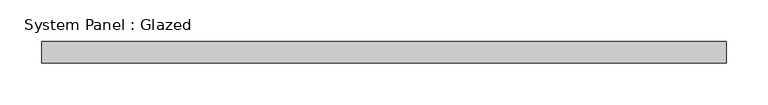
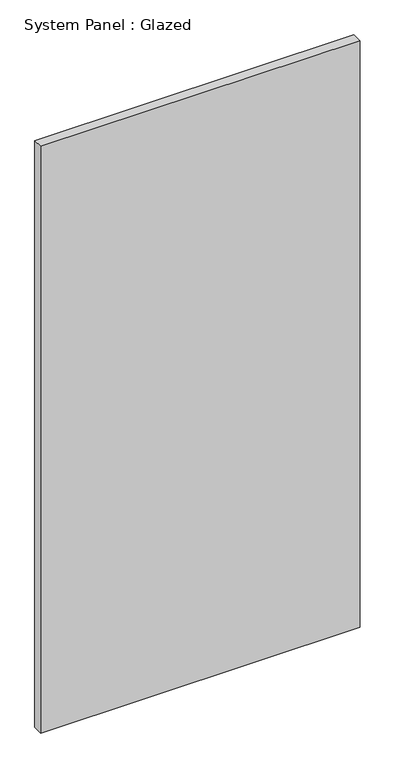
"""IFC4 building model written with IfcOpenShell, lengths in millimetres: plate geometry, System Panel : Glazed."""

from ifc_helpers import new_model, si_unit, origin, origin_with_axes, place, context, project, spatial, polyline, outline, extrude, source, transform, mapped, element, save


def system_panel_glazed_30877d7e(model_context):
    return source(origin(), model_context, "Body", "SweptSolid", [
        extrude(outline(polyline([(409.575, 19.05), (-409.575, 19.05), (-409.575, 44.45), (409.575, 44.45), (409.575, 19.05)])), origin_with_axes(), (0.0, 0.0, 1.0), 1590.1019301),
    ])


if __name__ == "__main__":
    model = new_model("IFC4")
    model_context = context("Model", 3, world=origin())
    ifc_project = project(units=[si_unit("LENGTHUNIT", "METRE", prefix="MILLI")], contexts=[model_context])
    site = spatial("IfcSite", under=ifc_project)
    building = spatial("IfcBuilding", under=site)
    placement = place(None, origin())
    system_panel_glazed_shape = system_panel_glazed_30877d7e(model_context)
    element("IfcPlate", 1, ObjectType="System Panel : Glazed", at=placement, inside=building, context=model_context, shape_type="MappedRepresentation", body=[
        mapped(system_panel_glazed_shape, transform((0.0, 0.0, 0.0), x_axis=(1.0, 0.0, 0.0), y_axis=(0.0, 1.0, 0.0), z_axis=(0.0, 0.0, 1.0))),
    ])
    save(model, "model.ifc")

# Revit data of these elements
# Type "System Panel : Glazed"
#   Construction Type Id = "GSP4R"
#   Analytic Construction = "1/8 in Pilkington single glazing"
#   Visual Light Transmittance = 0.9
#   Solar Heat Gain Coefficient = 0.86
#   Heat Transfer Coefficient (U) = 1.18115 BTU/(h·ft²·°F)
#   Define Thermal Properties by = 1
# Element 1 (IfcPlate, "System Panel : Glazed")
#   Materials on its faces: "Glass"
# Materials
#   "Glass": class "Glass", colour RGB 0 128 192, transparency 0.75, Description = "Soda Lime Glass", Cost = 0
